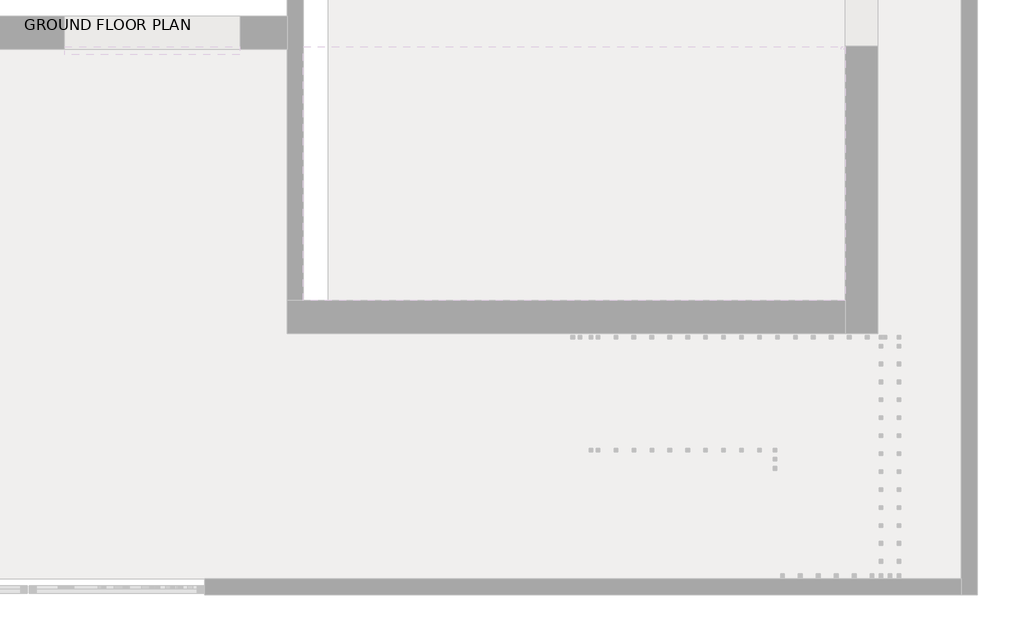
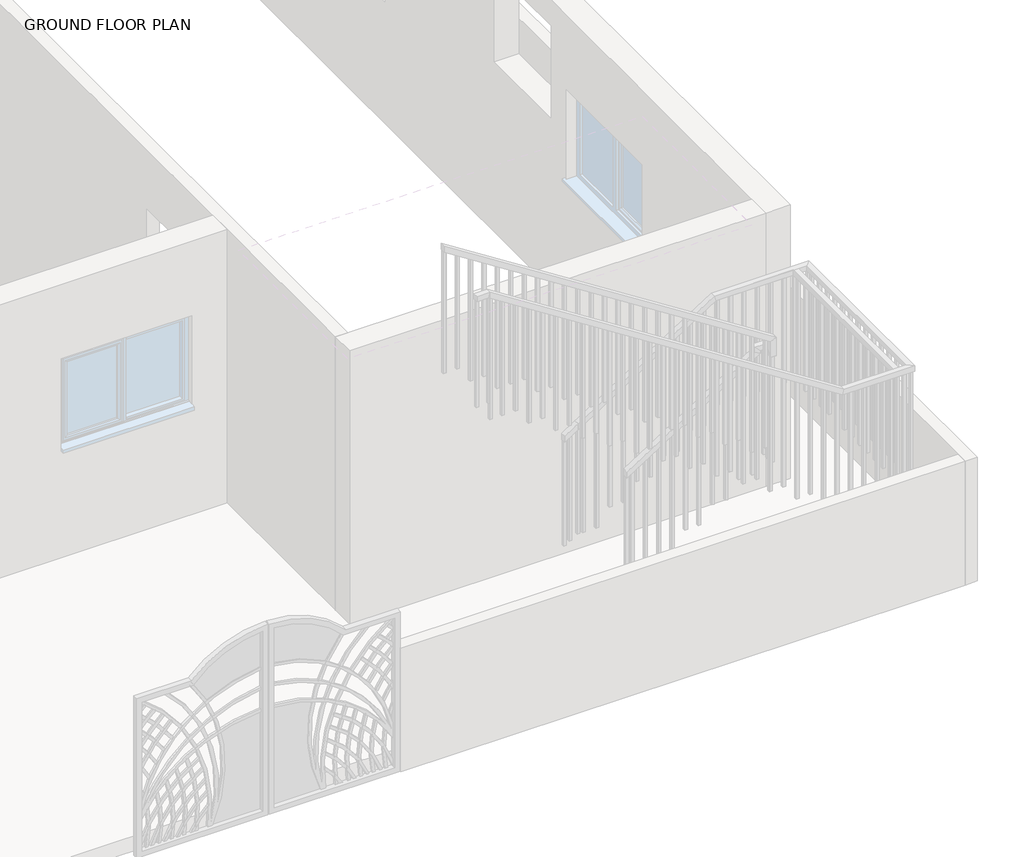
# One storey, part 21 of 23: 2 railings.
"""IFC4 building model written with IfcOpenShell, lengths in millimetres."""

from ifc_helpers import new_model, si_unit, frame, origin, place, context, project, spatial, polyline, outline, extrude, faceted_brep, element, save

model = new_model("IFC4")

# Units and contexts
model_context = context("Model", 3, world=origin())
ifc_project = project(units=[si_unit("LENGTHUNIT", "METRE", prefix="MILLI")], contexts=[model_context])

# Site, building, storey
site = spatial("IfcSite", under=ifc_project)
building = spatial("IfcBuilding", under=site)
storey = spatial("IfcBuildingStorey", under=building, Name="GROUND FLOOR PLAN", Elevation=487.68)

# Railings
placement = place(None, origin())
element("IfcRailing", 1, ObjectType="1100mm", at=placement, inside=storey, context=model_context, shape_type="SolidModel", body=[
    faceted_brep([(-8680.149573, -10220.0521308, 1912.8), (-8680.149573, -10220.0521308, 1853.4423995), (-8680.149573, -10270.0521308, 1853.4423995), (-8680.149573, -10270.0521308, 1912.8), (-7409.7306254, -10220.0521308, 2725.6), (-7395.1045513, -10220.0521308, 2675.6), (-7395.1045513, -10270.0521308, 2675.6), (-7409.7306254, -10270.0521308, 2725.6), (-6495.8132565, -10220.0521308, 2725.6), (-6495.8132565, -10220.0521308, 2675.6), (-6545.8132565, -10270.0521308, 2675.6), (-6545.8132565, -10270.0521308, 2725.6), (-6495.8132565, -11933.6860066, 2725.6), (-6495.8132565, -11933.6860066, 2675.6), (-6545.8132565, -11883.6860066, 2675.6), (-6545.8132565, -11883.6860066, 2725.6), (-7155.718398, -11933.6860066, 2725.6), (-7170.3479429, -11933.6860066, 2675.6), (-7170.3479429, -11883.6860066, 2675.6), (-7155.718398, -11883.6860066, 2725.6), (-10457.8773536, -11933.6860066, 4838.88), (-10457.8773536, -11883.6860066, 4838.88), (-10457.8773536, -11883.6860066, 4779.517542), (-10457.8773536, -11933.6860066, 4779.517542)], [[[0, 1, 2, 3]], [[1, 0, 4, 5]], [[2, 1, 5, 6]], [[3, 2, 6, 7]], [[0, 3, 7, 4]], [[5, 4, 8, 9]], [[6, 5, 9, 10]], [[7, 6, 10, 11]], [[4, 7, 11, 8]], [[9, 8, 12, 13]], [[10, 9, 13, 14]], [[11, 10, 14, 15]], [[8, 11, 15, 12]], [[13, 12, 16, 17]], [[14, 13, 17, 18]], [[15, 14, 18, 19]], [[12, 15, 19, 16]], [[20, 21, 22, 23]], [[17, 16, 20, 23]], [[18, 17, 23, 22]], [[19, 18, 22, 21]], [[16, 19, 21, 20]]]),
    extrude(outline(polyline([(4691.8007425, -10320.8132565), (4707.7999723, -10345.8132565), (3576.32, -10345.8132565), (3576.32, -10320.8132565), (4691.8007425, -10320.8132565)])), frame((0.0, -11921.1860066, 0.0), z_axis=(0.0, 1.0, 0.0), x_axis=(0.0, 0.0, 1.0)), (0.0, 0.0, 1.0), 25.0),
    extrude(outline(polyline([(4611.8045935, -10195.8132565), (4627.8038233, -10220.8132565), (3576.32, -10220.8132565), (3576.32, -10195.8132565), (4611.8045935, -10195.8132565)])), frame((0.0, -11921.1860066, 0.0), z_axis=(0.0, 1.0, 0.0), x_axis=(0.0, 0.0, 1.0)), (0.0, 0.0, 1.0), 25.0),
    extrude(outline(polyline([(4531.8084444, -10070.8132565), (4547.8076742, -10095.8132565), (3413.76, -10095.8132565), (3413.76, -10070.8132565), (4531.8084444, -10070.8132565)])), frame((0.0, -11921.1860066, 0.0), z_axis=(0.0, 1.0, 0.0), x_axis=(0.0, 0.0, 1.0)), (0.0, 0.0, 1.0), 25.0),
    extrude(outline(polyline([(4451.8122954, -9945.8132565), (4467.8115252, -9970.8132565), (3413.76, -9970.8132565), (3413.76, -9945.8132565), (4451.8122954, -9945.8132565)])), frame((0.0, -11921.1860066, 0.0), z_axis=(0.0, 1.0, 0.0), x_axis=(0.0, 0.0, 1.0)), (0.0, 0.0, 1.0), 25.0),
    extrude(outline(polyline([(4371.8161463, -9820.8132565), (4387.8153761, -9845.8132565), (3251.2, -9845.8132565), (3251.2, -9820.8132565), (4371.8161463, -9820.8132565)])), frame((0.0, -11921.1860066, 0.0), z_axis=(0.0, 1.0, 0.0), x_axis=(0.0, 0.0, 1.0)), (0.0, 0.0, 1.0), 25.0),
    extrude(outline(polyline([(4291.8423995, -9695.8132565), (4307.8371231, -9720.8132565), (3251.2, -9720.8132565), (3251.2, -9695.8132565), (4291.8423995, -9695.8132565)])), frame((0.0, -11921.1860066, 0.0), z_axis=(0.0, 1.0, 0.0), x_axis=(0.0, 0.0, 1.0)), (0.0, 0.0, 1.0), 25.0),
    extrude(outline(polyline([(4211.8238482, -9570.8132565), (4227.823078, -9595.8132565), (3088.64, -9595.8132565), (3088.64, -9570.8132565), (4211.8238482, -9570.8132565)])), frame((0.0, -11921.1860066, 0.0), z_axis=(0.0, 1.0, 0.0), x_axis=(0.0, 0.0, 1.0)), (0.0, 0.0, 1.0), 25.0),
    extrude(outline(polyline([(4131.8276992, -9445.8132565), (4147.826929, -9470.8132565), (3088.64, -9470.8132565), (3088.64, -9445.8132565), (4131.8276992, -9445.8132565)])), frame((0.0, -11921.1860066, 0.0), z_axis=(0.0, 1.0, 0.0), x_axis=(0.0, 0.0, 1.0)), (0.0, 0.0, 1.0), 25.0),
    extrude(outline(polyline([(4051.8315501, -9320.8132565), (4067.8307799, -9345.8132565), (2926.08, -9345.8132565), (2926.08, -9320.8132565), (4051.8315501, -9320.8132565)])), frame((0.0, -11921.1860066, 0.0), z_axis=(0.0, 1.0, 0.0), x_axis=(0.0, 0.0, 1.0)), (0.0, 0.0, 1.0), 25.0),
    extrude(outline(polyline([(3971.835401, -9195.8132565), (3987.8346309, -9220.8132565), (2926.08, -9220.8132565), (2926.08, -9195.8132565), (3971.835401, -9195.8132565)])), frame((0.0, -11921.1860066, 0.0), z_axis=(0.0, 1.0, 0.0), x_axis=(0.0, 0.0, 1.0)), (0.0, 0.0, 1.0), 25.0),
    extrude(outline(polyline([(3891.839252, -9070.8132565), (3907.8384818, -9095.8132565), (2763.52, -9095.8132565), (2763.52, -9070.8132565), (3891.839252, -9070.8132565)])), frame((0.0, -11921.1860066, 0.0), z_axis=(0.0, 1.0, 0.0), x_axis=(0.0, 0.0, 1.0)), (0.0, 0.0, 1.0), 25.0),
    extrude(outline(polyline([(3811.8431029, -8945.8132565), (3827.8423328, -8970.8132565), (2763.52, -8970.8132565), (2763.52, -8945.8132565), (3811.8431029, -8945.8132565)])), frame((0.0, -11921.1860066, 0.0), z_axis=(0.0, 1.0, 0.0), x_axis=(0.0, 0.0, 1.0)), (0.0, 0.0, 1.0), 25.0),
    extrude(outline(polyline([(3731.8469539, -8820.8132565), (3747.8461837, -8845.8132565), (2600.96, -8845.8132565), (2600.96, -8820.8132565), (3731.8469539, -8820.8132565)])), frame((0.0, -11921.1860066, 0.0), z_axis=(0.0, 1.0, 0.0), x_axis=(0.0, 0.0, 1.0)), (0.0, 0.0, 1.0), 25.0),
    extrude(outline(polyline([(3651.8508048, -8695.8132565), (3667.8500347, -8720.8132565), (2600.96, -8720.8132565), (2600.96, -8695.8132565), (3651.8508048, -8695.8132565)])), frame((0.0, -11921.1860066, 0.0), z_axis=(0.0, 1.0, 0.0), x_axis=(0.0, 0.0, 1.0)), (0.0, 0.0, 1.0), 25.0),
    extrude(outline(polyline([(3571.8546558, -8570.8132565), (3587.8538856, -8595.8132565), (2438.4, -8595.8132565), (2438.4, -8570.8132565), (3571.8546558, -8570.8132565)])), frame((0.0, -11921.1860066, 0.0), z_axis=(0.0, 1.0, 0.0), x_axis=(0.0, 0.0, 1.0)), (0.0, 0.0, 1.0), 25.0),
    extrude(outline(polyline([(3491.8585067, -8445.8132565), (3507.8577365, -8470.8132565), (2438.4, -8470.8132565), (2438.4, -8445.8132565), (3491.8585067, -8445.8132565)])), frame((0.0, -11921.1860066, 0.0), z_axis=(0.0, 1.0, 0.0), x_axis=(0.0, 0.0, 1.0)), (0.0, 0.0, 1.0), 25.0),
    extrude(outline(polyline([(3411.8623577, -8320.8132565), (3427.8615875, -8345.8132565), (2275.84, -8345.8132565), (2275.84, -8320.8132565), (3411.8623577, -8320.8132565)])), frame((0.0, -11921.1860066, 0.0), z_axis=(0.0, 1.0, 0.0), x_axis=(0.0, 0.0, 1.0)), (0.0, 0.0, 1.0), 25.0),
    extrude(outline(polyline([(3331.8662086, -8195.8132565), (3347.8654384, -8220.8132565), (2275.84, -8220.8132565), (2275.84, -8195.8132565), (3331.8662086, -8195.8132565)])), frame((0.0, -11921.1860066, 0.0), z_axis=(0.0, 1.0, 0.0), x_axis=(0.0, 0.0, 1.0)), (0.0, 0.0, 1.0), 25.0),
    extrude(outline(polyline([(3251.8700596, -8070.8132565), (3267.8692894, -8095.8132565), (2113.28, -8095.8132565), (2113.28, -8070.8132565), (3251.8700596, -8070.8132565)])), frame((0.0, -11921.1860066, 0.0), z_axis=(0.0, 1.0, 0.0), x_axis=(0.0, 0.0, 1.0)), (0.0, 0.0, 1.0), 25.0),
    extrude(outline(polyline([(3171.8739105, -7945.8132565), (3187.8731403, -7970.8132565), (2113.28, -7970.8132565), (2113.28, -7945.8132565), (3171.8739105, -7945.8132565)])), frame((0.0, -11921.1860066, 0.0), z_axis=(0.0, 1.0, 0.0), x_axis=(0.0, 0.0, 1.0)), (0.0, 0.0, 1.0), 25.0),
    extrude(outline(polyline([(3091.8777615, -7820.8132565), (3107.8769913, -7845.8132565), (1950.72, -7845.8132565), (1950.72, -7820.8132565), (3091.8777615, -7820.8132565)])), frame((0.0, -11921.1860066, 0.0), z_axis=(0.0, 1.0, 0.0), x_axis=(0.0, 0.0, 1.0)), (0.0, 0.0, 1.0), 25.0),
    extrude(outline(polyline([(3011.8816124, -7695.8132565), (3027.8808422, -7720.8132565), (1950.72, -7720.8132565), (1950.72, -7695.8132565), (3011.8816124, -7695.8132565)])), frame((0.0, -11921.1860066, 0.0), z_axis=(0.0, 1.0, 0.0), x_axis=(0.0, 0.0, 1.0)), (0.0, 0.0, 1.0), 25.0),
    extrude(outline(polyline([(2931.8854634, -7570.8132565), (2947.8846932, -7595.8132565), (1788.16, -7595.8132565), (1788.16, -7570.8132565), (2931.8854634, -7570.8132565)])), frame((0.0, -11921.1860066, 0.0), z_axis=(0.0, 1.0, 0.0), x_axis=(0.0, 0.0, 1.0)), (0.0, 0.0, 1.0), 25.0),
    extrude(outline(polyline([(2851.8893143, -7445.8132565), (2867.8885441, -7470.8132565), (1788.16, -7470.8132565), (1788.16, -7445.8132565), (2851.8893143, -7445.8132565)])), frame((0.0, -11921.1860066, 0.0), z_axis=(0.0, 1.0, 0.0), x_axis=(0.0, 0.0, 1.0)), (0.0, 0.0, 1.0), 25.0),
    extrude(outline(polyline([(2771.8931653, -7320.8132565), (2787.8923951, -7345.8132565), (1625.6, -7345.8132565), (1625.6, -7320.8132565), (2771.8931653, -7320.8132565)])), frame((0.0, -11921.1860066, 0.0), z_axis=(0.0, 1.0, 0.0), x_axis=(0.0, 0.0, 1.0)), (0.0, 0.0, 1.0), 25.0),
    extrude(outline(polyline([(2691.8970162, -7195.8132565), (2707.896246, -7220.8132565), (1625.6, -7220.8132565), (1625.6, -7195.8132565), (2691.8970162, -7195.8132565)])), frame((0.0, -11921.1860066, 0.0), z_axis=(0.0, 1.0, 0.0), x_axis=(0.0, 0.0, 1.0)), (0.0, 0.0, 1.0), 25.0),
    extrude(outline(polyline([(-7070.8132565, -11921.1860066), (-7095.8132565, -11921.1860066), (-7095.8132565, -11896.1860066), (-7070.8132565, -11896.1860066), (-7070.8132565, -11921.1860066)])), frame((0.0, 0.0, 1625.6), z_axis=(0.0, 0.0, 1.0), x_axis=(1.0, 0.0, 0.0)), (0.0, 0.0, 1.0), 1050.0),
    extrude(outline(polyline([(-6945.8132565, -11921.1860066), (-6970.8132565, -11921.1860066), (-6970.8132565, -11896.1860066), (-6945.8132565, -11896.1860066), (-6945.8132565, -11921.1860066)])), frame((0.0, 0.0, 1625.6), z_axis=(0.0, 0.0, 1.0), x_axis=(1.0, 0.0, 0.0)), (0.0, 0.0, 1.0), 1050.0),
    extrude(outline(polyline([(-6820.8132565, -11921.1860066), (-6845.8132565, -11921.1860066), (-6845.8132565, -11896.1860066), (-6820.8132565, -11896.1860066), (-6820.8132565, -11921.1860066)])), frame((0.0, 0.0, 1625.6), z_axis=(0.0, 0.0, 1.0), x_axis=(1.0, 0.0, 0.0)), (0.0, 0.0, 1.0), 1050.0),
    extrude(outline(polyline([(-6695.8132565, -11921.1860066), (-6720.8132565, -11921.1860066), (-6720.8132565, -11896.1860066), (-6695.8132565, -11896.1860066), (-6695.8132565, -11921.1860066)])), frame((0.0, 0.0, 1625.6), z_axis=(0.0, 0.0, 1.0), x_axis=(1.0, 0.0, 0.0)), (0.0, 0.0, 1.0), 1050.0),
    extrude(outline(polyline([(-6570.8132565, -11921.1860066), (-6595.8132565, -11921.1860066), (-6595.8132565, -11896.1860066), (-6570.8132565, -11896.1860066), (-6570.8132565, -11921.1860066)])), frame((0.0, 0.0, 1625.6), z_axis=(0.0, 0.0, 1.0), x_axis=(1.0, 0.0, 0.0)), (0.0, 0.0, 1.0), 1050.0),
    extrude(outline(polyline([(-6508.3132565, -11795.0521308), (-6508.3132565, -11820.0521308), (-6533.3132565, -11820.0521308), (-6533.3132565, -11795.0521308), (-6508.3132565, -11795.0521308)])), frame((0.0, 0.0, 1625.6), z_axis=(0.0, 0.0, 1.0), x_axis=(1.0, 0.0, 0.0)), (0.0, 0.0, 1.0), 1050.0),
    extrude(outline(polyline([(-6508.3132565, -11670.0521308), (-6508.3132565, -11695.0521308), (-6533.3132565, -11695.0521308), (-6533.3132565, -11670.0521308), (-6508.3132565, -11670.0521308)])), frame((0.0, 0.0, 1625.6), z_axis=(0.0, 0.0, 1.0), x_axis=(1.0, 0.0, 0.0)), (0.0, 0.0, 1.0), 1050.0),
    extrude(outline(polyline([(-6508.3132565, -11545.0521308), (-6508.3132565, -11570.0521308), (-6533.3132565, -11570.0521308), (-6533.3132565, -11545.0521308), (-6508.3132565, -11545.0521308)])), frame((0.0, 0.0, 1625.6), z_axis=(0.0, 0.0, 1.0), x_axis=(1.0, 0.0, 0.0)), (0.0, 0.0, 1.0), 1050.0),
    extrude(outline(polyline([(-6508.3132565, -11420.0521308), (-6508.3132565, -11445.0521308), (-6533.3132565, -11445.0521308), (-6533.3132565, -11420.0521308), (-6508.3132565, -11420.0521308)])), frame((0.0, 0.0, 1625.6), z_axis=(0.0, 0.0, 1.0), x_axis=(1.0, 0.0, 0.0)), (0.0, 0.0, 1.0), 1050.0),
    extrude(outline(polyline([(-6508.3132565, -11295.0521308), (-6508.3132565, -11320.0521308), (-6533.3132565, -11320.0521308), (-6533.3132565, -11295.0521308), (-6508.3132565, -11295.0521308)])), frame((0.0, 0.0, 1625.6), z_axis=(0.0, 0.0, 1.0), x_axis=(1.0, 0.0, 0.0)), (0.0, 0.0, 1.0), 1050.0),
    extrude(outline(polyline([(-6508.3132565, -11170.0521308), (-6508.3132565, -11195.0521308), (-6533.3132565, -11195.0521308), (-6533.3132565, -11170.0521308), (-6508.3132565, -11170.0521308)])), frame((0.0, 0.0, 1625.6), z_axis=(0.0, 0.0, 1.0), x_axis=(1.0, 0.0, 0.0)), (0.0, 0.0, 1.0), 1050.0),
    extrude(outline(polyline([(-6508.3132565, -11045.0521308), (-6508.3132565, -11070.0521308), (-6533.3132565, -11070.0521308), (-6533.3132565, -11045.0521308), (-6508.3132565, -11045.0521308)])), frame((0.0, 0.0, 1625.6), z_axis=(0.0, 0.0, 1.0), x_axis=(1.0, 0.0, 0.0)), (0.0, 0.0, 1.0), 1050.0),
    extrude(outline(polyline([(-6508.3132565, -10920.0521308), (-6508.3132565, -10945.0521308), (-6533.3132565, -10945.0521308), (-6533.3132565, -10920.0521308), (-6508.3132565, -10920.0521308)])), frame((0.0, 0.0, 1625.6), z_axis=(0.0, 0.0, 1.0), x_axis=(1.0, 0.0, 0.0)), (0.0, 0.0, 1.0), 1050.0),
    extrude(outline(polyline([(-6508.3132565, -10795.0521308), (-6508.3132565, -10820.0521308), (-6533.3132565, -10820.0521308), (-6533.3132565, -10795.0521308), (-6508.3132565, -10795.0521308)])), frame((0.0, 0.0, 1625.6), z_axis=(0.0, 0.0, 1.0), x_axis=(1.0, 0.0, 0.0)), (0.0, 0.0, 1.0), 1050.0),
    extrude(outline(polyline([(-6508.3132565, -10670.0521308), (-6508.3132565, -10695.0521308), (-6533.3132565, -10695.0521308), (-6533.3132565, -10670.0521308), (-6508.3132565, -10670.0521308)])), frame((0.0, 0.0, 1625.6), z_axis=(0.0, 0.0, 1.0), x_axis=(1.0, 0.0, 0.0)), (0.0, 0.0, 1.0), 1050.0),
    extrude(outline(polyline([(-6508.3132565, -10545.0521308), (-6508.3132565, -10570.0521308), (-6533.3132565, -10570.0521308), (-6533.3132565, -10545.0521308), (-6508.3132565, -10545.0521308)])), frame((0.0, 0.0, 1625.6), z_axis=(0.0, 0.0, 1.0), x_axis=(1.0, 0.0, 0.0)), (0.0, 0.0, 1.0), 1050.0),
    extrude(outline(polyline([(-6508.3132565, -10420.0521308), (-6508.3132565, -10445.0521308), (-6533.3132565, -10445.0521308), (-6533.3132565, -10420.0521308), (-6508.3132565, -10420.0521308)])), frame((0.0, 0.0, 1625.6), z_axis=(0.0, 0.0, 1.0), x_axis=(1.0, 0.0, 0.0)), (0.0, 0.0, 1.0), 1050.0),
    extrude(outline(polyline([(-6508.3132565, -10295.0521308), (-6508.3132565, -10320.0521308), (-6533.3132565, -10320.0521308), (-6533.3132565, -10295.0521308), (-6508.3132565, -10295.0521308)])), frame((0.0, 0.0, 1625.6), z_axis=(0.0, 0.0, 1.0), x_axis=(1.0, 0.0, 0.0)), (0.0, 0.0, 1.0), 1050.0),
    extrude(outline(polyline([(-6630.149573, -10232.5521308), (-6605.149573, -10232.5521308), (-6605.149573, -10257.5521308), (-6630.149573, -10257.5521308), (-6630.149573, -10232.5521308)])), frame((0.0, 0.0, 1625.6), z_axis=(0.0, 0.0, 1.0), x_axis=(1.0, 0.0, 0.0)), (0.0, 0.0, 1.0), 1050.0),
    extrude(outline(polyline([(-6755.149573, -10232.5521308), (-6730.149573, -10232.5521308), (-6730.149573, -10257.5521308), (-6755.149573, -10257.5521308), (-6755.149573, -10232.5521308)])), frame((0.0, 0.0, 1625.6), z_axis=(0.0, 0.0, 1.0), x_axis=(1.0, 0.0, 0.0)), (0.0, 0.0, 1.0), 1050.0),
    extrude(outline(polyline([(-6880.149573, -10232.5521308), (-6855.149573, -10232.5521308), (-6855.149573, -10257.5521308), (-6880.149573, -10257.5521308), (-6880.149573, -10232.5521308)])), frame((0.0, 0.0, 1625.6), z_axis=(0.0, 0.0, 1.0), x_axis=(1.0, 0.0, 0.0)), (0.0, 0.0, 1.0), 1050.0),
    extrude(outline(polyline([(-7005.149573, -10232.5521308), (-6980.149573, -10232.5521308), (-6980.149573, -10257.5521308), (-7005.149573, -10257.5521308), (-7005.149573, -10232.5521308)])), frame((0.0, 0.0, 1625.6), z_axis=(0.0, 0.0, 1.0), x_axis=(1.0, 0.0, 0.0)), (0.0, 0.0, 1.0), 1050.0),
    extrude(outline(polyline([(-7130.149573, -10232.5521308), (-7105.149573, -10232.5521308), (-7105.149573, -10257.5521308), (-7130.149573, -10257.5521308), (-7130.149573, -10232.5521308)])), frame((0.0, 0.0, 1625.6), z_axis=(0.0, 0.0, 1.0), x_axis=(1.0, 0.0, 0.0)), (0.0, 0.0, 1.0), 1050.0),
    extrude(outline(polyline([(-7255.149573, -10232.5521308), (-7230.149573, -10232.5521308), (-7230.149573, -10257.5521308), (-7255.149573, -10257.5521308), (-7255.149573, -10232.5521308)])), frame((0.0, 0.0, 1625.6), z_axis=(0.0, 0.0, 1.0), x_axis=(1.0, 0.0, 0.0)), (0.0, 0.0, 1.0), 1050.0),
    extrude(outline(polyline([(-7380.149573, -10232.5521308), (-7355.149573, -10232.5521308), (-7355.149573, -10257.5521308), (-7380.149573, -10257.5521308), (-7380.149573, -10232.5521308)])), frame((0.0, 0.0, 1625.6), z_axis=(0.0, 0.0, 1.0), x_axis=(1.0, 0.0, 0.0)), (0.0, 0.0, 1.0), 1050.0),
    extrude(outline(polyline([(1463.04, -7505.149573), (1463.04, -7480.149573), (2621.1891352, -7480.149573), (2605.1944115, -7505.149573), (1463.04, -7505.149573)])), frame((0.0, -10257.5521308, 0.0), z_axis=(0.0, 1.0, 0.0), x_axis=(0.0, 0.0, 1.0)), (0.0, 0.0, 1.0), 25.0),
    extrude(outline(polyline([(1463.04, -7630.149573), (1463.04, -7605.149573), (2541.2155169, -7605.149573), (2525.2207932, -7630.149573), (1463.04, -7630.149573)])), frame((0.0, -10257.5521308, 0.0), z_axis=(0.0, 1.0, 0.0), x_axis=(0.0, 0.0, 1.0)), (0.0, 0.0, 1.0), 25.0),
    extrude(outline(polyline([(1300.48, -7755.149573), (1300.48, -7730.149573), (2461.2418986, -7730.149573), (2445.2471749, -7755.149573), (1300.48, -7755.149573)])), frame((0.0, -10257.5521308, 0.0), z_axis=(0.0, 1.0, 0.0), x_axis=(0.0, 0.0, 1.0)), (0.0, 0.0, 1.0), 25.0),
    extrude(outline(polyline([(1300.48, -7880.149573), (1300.48, -7855.149573), (2381.2682803, -7855.149573), (2365.2735566, -7880.149573), (1300.48, -7880.149573)])), frame((0.0, -10257.5521308, 0.0), z_axis=(0.0, 1.0, 0.0), x_axis=(0.0, 0.0, 1.0)), (0.0, 0.0, 1.0), 25.0),
    extrude(outline(polyline([(1137.92, -8005.149573), (1137.92, -7980.149573), (2301.294662, -7980.149573), (2285.2999383, -8005.149573), (1137.92, -8005.149573)])), frame((0.0, -10257.5521308, 0.0), z_axis=(0.0, 1.0, 0.0), x_axis=(0.0, 0.0, 1.0)), (0.0, 0.0, 1.0), 25.0),
    extrude(outline(polyline([(1137.92, -8130.149573), (1137.92, -8105.149573), (2221.3210437, -8105.149573), (2205.32632, -8130.149573), (1137.92, -8130.149573)])), frame((0.0, -10257.5521308, 0.0), z_axis=(0.0, 1.0, 0.0), x_axis=(0.0, 0.0, 1.0)), (0.0, 0.0, 1.0), 25.0),
    extrude(outline(polyline([(975.36, -8255.149573), (975.36, -8230.149573), (2141.3474254, -8230.149573), (2125.3527017, -8255.149573), (975.36, -8255.149573)])), frame((0.0, -10257.5521308, 0.0), z_axis=(0.0, 1.0, 0.0), x_axis=(0.0, 0.0, 1.0)), (0.0, 0.0, 1.0), 25.0),
    extrude(outline(polyline([(975.36, -8380.149573), (975.36, -8355.149573), (2061.3738071, -8355.149573), (2045.3790834, -8380.149573), (975.36, -8380.149573)])), frame((0.0, -10257.5521308, 0.0), z_axis=(0.0, 1.0, 0.0), x_axis=(0.0, 0.0, 1.0)), (0.0, 0.0, 1.0), 25.0),
    extrude(outline(polyline([(812.8, -8505.149573), (812.8, -8480.149573), (1981.4001888, -8480.149573), (1965.4054651, -8505.149573), (812.8, -8505.149573)])), frame((0.0, -10257.5521308, 0.0), z_axis=(0.0, 1.0, 0.0), x_axis=(0.0, 0.0, 1.0)), (0.0, 0.0, 1.0), 25.0),
    extrude(outline(polyline([(812.8, -8630.149573), (812.8, -8605.149573), (1901.4265705, -8605.149573), (1885.4318468, -8630.149573), (812.8, -8630.149573)])), frame((0.0, -10257.5521308, 0.0), z_axis=(0.0, 1.0, 0.0), x_axis=(0.0, 0.0, 1.0)), (0.0, 0.0, 1.0), 25.0),
    extrude(outline(polyline([(-6508.3132565, -11896.1860066), (-6508.3132565, -11921.1860066), (-6533.3132565, -11921.1860066), (-6533.3132565, -11896.1860066), (-6508.3132565, -11896.1860066)])), frame((0.0, 0.0, 1625.6), z_axis=(0.0, 0.0, 1.0), x_axis=(1.0, 0.0, 0.0)), (0.0, 0.0, 1.0), 1050.0),
    extrude(outline(polyline([(-6533.3132565, -10232.5521308), (-6508.3132565, -10232.5521308), (-6508.3132565, -10257.5521308), (-6533.3132565, -10257.5521308), (-6533.3132565, -10232.5521308)])), frame((0.0, 0.0, 1625.6), z_axis=(0.0, 0.0, 1.0), x_axis=(1.0, 0.0, 0.0)), (0.0, 0.0, 1.0), 1050.0),
    extrude(outline(polyline([(4763.5183122, -10432.8773536), (4779.517542, -10457.8773536), (3576.32, -10457.8773536), (3576.32, -10432.8773536), (4763.5183122, -10432.8773536)])), frame((0.0, -11921.1860066, 0.0), z_axis=(0.0, 1.0, 0.0), x_axis=(0.0, 0.0, 1.0)), (0.0, 0.0, 1.0), 25.0),
    extrude(outline(polyline([(812.8, -8680.149573), (812.8, -8655.149573), (1869.4371231, -8655.149573), (1853.4423995, -8680.149573), (812.8, -8680.149573)])), frame((0.0, -10257.5521308, 0.0), z_axis=(0.0, 1.0, 0.0), x_axis=(0.0, 0.0, 1.0)), (0.0, 0.0, 1.0), 25.0),
])
element("IfcRailing", 2, ObjectType="1100mm", at=placement, inside=storey, context=model_context, shape_type="SolidModel", body=[
    faceted_brep([(-8680.149573, -10220.0521308, 1912.8), (-8680.149573, -10220.0521308, 1853.4423995), (-8680.149573, -10270.0521308, 1853.4423995), (-8680.149573, -10270.0521308, 1912.8), (-7409.7306254, -10220.0521308, 2725.6), (-7395.1045513, -10220.0521308, 2675.6), (-7395.1045513, -10270.0521308, 2675.6), (-7409.7306254, -10270.0521308, 2725.6), (-6495.8132565, -10220.0521308, 2725.6), (-6495.8132565, -10220.0521308, 2675.6), (-6545.8132565, -10270.0521308, 2675.6), (-6545.8132565, -10270.0521308, 2725.6), (-6495.8132565, -11933.6860066, 2725.6), (-6495.8132565, -11933.6860066, 2675.6), (-6545.8132565, -11883.6860066, 2675.6), (-6545.8132565, -11883.6860066, 2725.6), (-7155.718398, -11933.6860066, 2725.6), (-7170.3479429, -11933.6860066, 2675.6), (-7170.3479429, -11883.6860066, 2675.6), (-7155.718398, -11883.6860066, 2725.6), (-10457.8773536, -11933.6860066, 4838.88), (-10457.8773536, -11883.6860066, 4838.88), (-10457.8773536, -11883.6860066, 4779.517542), (-10457.8773536, -11933.6860066, 4779.517542)], [[[0, 1, 2, 3]], [[1, 0, 4, 5]], [[2, 1, 5, 6]], [[3, 2, 6, 7]], [[0, 3, 7, 4]], [[5, 4, 8, 9]], [[6, 5, 9, 10]], [[7, 6, 10, 11]], [[4, 7, 11, 8]], [[9, 8, 12, 13]], [[10, 9, 13, 14]], [[11, 10, 14, 15]], [[8, 11, 15, 12]], [[13, 12, 16, 17]], [[14, 13, 17, 18]], [[15, 14, 18, 19]], [[12, 15, 19, 16]], [[20, 21, 22, 23]], [[17, 16, 20, 23]], [[18, 17, 23, 22]], [[19, 18, 22, 21]], [[16, 19, 21, 20]]]),
    extrude(outline(polyline([(4691.8007425, -10320.8132565), (4707.7999723, -10345.8132565), (3576.32, -10345.8132565), (3576.32, -10320.8132565), (4691.8007425, -10320.8132565)])), frame((0.0, -11921.1860066, 0.0), z_axis=(0.0, 1.0, 0.0), x_axis=(0.0, 0.0, 1.0)), (0.0, 0.0, 1.0), 25.0),
    extrude(outline(polyline([(4611.8045935, -10195.8132565), (4627.8038233, -10220.8132565), (3576.32, -10220.8132565), (3576.32, -10195.8132565), (4611.8045935, -10195.8132565)])), frame((0.0, -11921.1860066, 0.0), z_axis=(0.0, 1.0, 0.0), x_axis=(0.0, 0.0, 1.0)), (0.0, 0.0, 1.0), 25.0),
    extrude(outline(polyline([(4531.8084444, -10070.8132565), (4547.8076742, -10095.8132565), (3413.76, -10095.8132565), (3413.76, -10070.8132565), (4531.8084444, -10070.8132565)])), frame((0.0, -11921.1860066, 0.0), z_axis=(0.0, 1.0, 0.0), x_axis=(0.0, 0.0, 1.0)), (0.0, 0.0, 1.0), 25.0),
    extrude(outline(polyline([(4451.8122954, -9945.8132565), (4467.8115252, -9970.8132565), (3413.76, -9970.8132565), (3413.76, -9945.8132565), (4451.8122954, -9945.8132565)])), frame((0.0, -11921.1860066, 0.0), z_axis=(0.0, 1.0, 0.0), x_axis=(0.0, 0.0, 1.0)), (0.0, 0.0, 1.0), 25.0),
    extrude(outline(polyline([(4371.8161463, -9820.8132565), (4387.8153761, -9845.8132565), (3251.2, -9845.8132565), (3251.2, -9820.8132565), (4371.8161463, -9820.8132565)])), frame((0.0, -11921.1860066, 0.0), z_axis=(0.0, 1.0, 0.0), x_axis=(0.0, 0.0, 1.0)), (0.0, 0.0, 1.0), 25.0),
    extrude(outline(polyline([(4291.8423995, -9695.8132565), (4307.8371231, -9720.8132565), (3251.2, -9720.8132565), (3251.2, -9695.8132565), (4291.8423995, -9695.8132565)])), frame((0.0, -11921.1860066, 0.0), z_axis=(0.0, 1.0, 0.0), x_axis=(0.0, 0.0, 1.0)), (0.0, 0.0, 1.0), 25.0),
    extrude(outline(polyline([(4211.8238482, -9570.8132565), (4227.823078, -9595.8132565), (3088.64, -9595.8132565), (3088.64, -9570.8132565), (4211.8238482, -9570.8132565)])), frame((0.0, -11921.1860066, 0.0), z_axis=(0.0, 1.0, 0.0), x_axis=(0.0, 0.0, 1.0)), (0.0, 0.0, 1.0), 25.0),
    extrude(outline(polyline([(4131.8276992, -9445.8132565), (4147.826929, -9470.8132565), (3088.64, -9470.8132565), (3088.64, -9445.8132565), (4131.8276992, -9445.8132565)])), frame((0.0, -11921.1860066, 0.0), z_axis=(0.0, 1.0, 0.0), x_axis=(0.0, 0.0, 1.0)), (0.0, 0.0, 1.0), 25.0),
    extrude(outline(polyline([(4051.8315501, -9320.8132565), (4067.8307799, -9345.8132565), (2926.08, -9345.8132565), (2926.08, -9320.8132565), (4051.8315501, -9320.8132565)])), frame((0.0, -11921.1860066, 0.0), z_axis=(0.0, 1.0, 0.0), x_axis=(0.0, 0.0, 1.0)), (0.0, 0.0, 1.0), 25.0),
    extrude(outline(polyline([(3971.835401, -9195.8132565), (3987.8346309, -9220.8132565), (2926.08, -9220.8132565), (2926.08, -9195.8132565), (3971.835401, -9195.8132565)])), frame((0.0, -11921.1860066, 0.0), z_axis=(0.0, 1.0, 0.0), x_axis=(0.0, 0.0, 1.0)), (0.0, 0.0, 1.0), 25.0),
    extrude(outline(polyline([(3891.839252, -9070.8132565), (3907.8384818, -9095.8132565), (2763.52, -9095.8132565), (2763.52, -9070.8132565), (3891.839252, -9070.8132565)])), frame((0.0, -11921.1860066, 0.0), z_axis=(0.0, 1.0, 0.0), x_axis=(0.0, 0.0, 1.0)), (0.0, 0.0, 1.0), 25.0),
    extrude(outline(polyline([(3811.8431029, -8945.8132565), (3827.8423328, -8970.8132565), (2763.52, -8970.8132565), (2763.52, -8945.8132565), (3811.8431029, -8945.8132565)])), frame((0.0, -11921.1860066, 0.0), z_axis=(0.0, 1.0, 0.0), x_axis=(0.0, 0.0, 1.0)), (0.0, 0.0, 1.0), 25.0),
    extrude(outline(polyline([(3731.8469539, -8820.8132565), (3747.8461837, -8845.8132565), (2600.96, -8845.8132565), (2600.96, -8820.8132565), (3731.8469539, -8820.8132565)])), frame((0.0, -11921.1860066, 0.0), z_axis=(0.0, 1.0, 0.0), x_axis=(0.0, 0.0, 1.0)), (0.0, 0.0, 1.0), 25.0),
    extrude(outline(polyline([(3651.8508048, -8695.8132565), (3667.8500347, -8720.8132565), (2600.96, -8720.8132565), (2600.96, -8695.8132565), (3651.8508048, -8695.8132565)])), frame((0.0, -11921.1860066, 0.0), z_axis=(0.0, 1.0, 0.0), x_axis=(0.0, 0.0, 1.0)), (0.0, 0.0, 1.0), 25.0),
    extrude(outline(polyline([(3571.8546558, -8570.8132565), (3587.8538856, -8595.8132565), (2438.4, -8595.8132565), (2438.4, -8570.8132565), (3571.8546558, -8570.8132565)])), frame((0.0, -11921.1860066, 0.0), z_axis=(0.0, 1.0, 0.0), x_axis=(0.0, 0.0, 1.0)), (0.0, 0.0, 1.0), 25.0),
    extrude(outline(polyline([(3491.8585067, -8445.8132565), (3507.8577365, -8470.8132565), (2438.4, -8470.8132565), (2438.4, -8445.8132565), (3491.8585067, -8445.8132565)])), frame((0.0, -11921.1860066, 0.0), z_axis=(0.0, 1.0, 0.0), x_axis=(0.0, 0.0, 1.0)), (0.0, 0.0, 1.0), 25.0),
    extrude(outline(polyline([(3411.8623577, -8320.8132565), (3427.8615875, -8345.8132565), (2275.84, -8345.8132565), (2275.84, -8320.8132565), (3411.8623577, -8320.8132565)])), frame((0.0, -11921.1860066, 0.0), z_axis=(0.0, 1.0, 0.0), x_axis=(0.0, 0.0, 1.0)), (0.0, 0.0, 1.0), 25.0),
    extrude(outline(polyline([(3331.8662086, -8195.8132565), (3347.8654384, -8220.8132565), (2275.84, -8220.8132565), (2275.84, -8195.8132565), (3331.8662086, -8195.8132565)])), frame((0.0, -11921.1860066, 0.0), z_axis=(0.0, 1.0, 0.0), x_axis=(0.0, 0.0, 1.0)), (0.0, 0.0, 1.0), 25.0),
    extrude(outline(polyline([(3251.8700596, -8070.8132565), (3267.8692894, -8095.8132565), (2113.28, -8095.8132565), (2113.28, -8070.8132565), (3251.8700596, -8070.8132565)])), frame((0.0, -11921.1860066, 0.0), z_axis=(0.0, 1.0, 0.0), x_axis=(0.0, 0.0, 1.0)), (0.0, 0.0, 1.0), 25.0),
    extrude(outline(polyline([(3171.8739105, -7945.8132565), (3187.8731403, -7970.8132565), (2113.28, -7970.8132565), (2113.28, -7945.8132565), (3171.8739105, -7945.8132565)])), frame((0.0, -11921.1860066, 0.0), z_axis=(0.0, 1.0, 0.0), x_axis=(0.0, 0.0, 1.0)), (0.0, 0.0, 1.0), 25.0),
    extrude(outline(polyline([(3091.8777615, -7820.8132565), (3107.8769913, -7845.8132565), (1950.72, -7845.8132565), (1950.72, -7820.8132565), (3091.8777615, -7820.8132565)])), frame((0.0, -11921.1860066, 0.0), z_axis=(0.0, 1.0, 0.0), x_axis=(0.0, 0.0, 1.0)), (0.0, 0.0, 1.0), 25.0),
    extrude(outline(polyline([(3011.8816124, -7695.8132565), (3027.8808422, -7720.8132565), (1950.72, -7720.8132565), (1950.72, -7695.8132565), (3011.8816124, -7695.8132565)])), frame((0.0, -11921.1860066, 0.0), z_axis=(0.0, 1.0, 0.0), x_axis=(0.0, 0.0, 1.0)), (0.0, 0.0, 1.0), 25.0),
    extrude(outline(polyline([(2931.8854634, -7570.8132565), (2947.8846932, -7595.8132565), (1788.16, -7595.8132565), (1788.16, -7570.8132565), (2931.8854634, -7570.8132565)])), frame((0.0, -11921.1860066, 0.0), z_axis=(0.0, 1.0, 0.0), x_axis=(0.0, 0.0, 1.0)), (0.0, 0.0, 1.0), 25.0),
    extrude(outline(polyline([(2851.8893143, -7445.8132565), (2867.8885441, -7470.8132565), (1788.16, -7470.8132565), (1788.16, -7445.8132565), (2851.8893143, -7445.8132565)])), frame((0.0, -11921.1860066, 0.0), z_axis=(0.0, 1.0, 0.0), x_axis=(0.0, 0.0, 1.0)), (0.0, 0.0, 1.0), 25.0),
    extrude(outline(polyline([(2771.8931653, -7320.8132565), (2787.8923951, -7345.8132565), (1625.6, -7345.8132565), (1625.6, -7320.8132565), (2771.8931653, -7320.8132565)])), frame((0.0, -11921.1860066, 0.0), z_axis=(0.0, 1.0, 0.0), x_axis=(0.0, 0.0, 1.0)), (0.0, 0.0, 1.0), 25.0),
    extrude(outline(polyline([(2691.8970162, -7195.8132565), (2707.896246, -7220.8132565), (1625.6, -7220.8132565), (1625.6, -7195.8132565), (2691.8970162, -7195.8132565)])), frame((0.0, -11921.1860066, 0.0), z_axis=(0.0, 1.0, 0.0), x_axis=(0.0, 0.0, 1.0)), (0.0, 0.0, 1.0), 25.0),
    extrude(outline(polyline([(-7070.8132565, -11921.1860066), (-7095.8132565, -11921.1860066), (-7095.8132565, -11896.1860066), (-7070.8132565, -11896.1860066), (-7070.8132565, -11921.1860066)])), frame((0.0, 0.0, 1625.6), z_axis=(0.0, 0.0, 1.0), x_axis=(1.0, 0.0, 0.0)), (0.0, 0.0, 1.0), 1050.0),
    extrude(outline(polyline([(-6945.8132565, -11921.1860066), (-6970.8132565, -11921.1860066), (-6970.8132565, -11896.1860066), (-6945.8132565, -11896.1860066), (-6945.8132565, -11921.1860066)])), frame((0.0, 0.0, 1625.6), z_axis=(0.0, 0.0, 1.0), x_axis=(1.0, 0.0, 0.0)), (0.0, 0.0, 1.0), 1050.0),
    extrude(outline(polyline([(-6820.8132565, -11921.1860066), (-6845.8132565, -11921.1860066), (-6845.8132565, -11896.1860066), (-6820.8132565, -11896.1860066), (-6820.8132565, -11921.1860066)])), frame((0.0, 0.0, 1625.6), z_axis=(0.0, 0.0, 1.0), x_axis=(1.0, 0.0, 0.0)), (0.0, 0.0, 1.0), 1050.0),
    extrude(outline(polyline([(-6695.8132565, -11921.1860066), (-6720.8132565, -11921.1860066), (-6720.8132565, -11896.1860066), (-6695.8132565, -11896.1860066), (-6695.8132565, -11921.1860066)])), frame((0.0, 0.0, 1625.6), z_axis=(0.0, 0.0, 1.0), x_axis=(1.0, 0.0, 0.0)), (0.0, 0.0, 1.0), 1050.0),
    extrude(outline(polyline([(-6570.8132565, -11921.1860066), (-6595.8132565, -11921.1860066), (-6595.8132565, -11896.1860066), (-6570.8132565, -11896.1860066), (-6570.8132565, -11921.1860066)])), frame((0.0, 0.0, 1625.6), z_axis=(0.0, 0.0, 1.0), x_axis=(1.0, 0.0, 0.0)), (0.0, 0.0, 1.0), 1050.0),
    extrude(outline(polyline([(-6508.3132565, -11795.0521308), (-6508.3132565, -11820.0521308), (-6533.3132565, -11820.0521308), (-6533.3132565, -11795.0521308), (-6508.3132565, -11795.0521308)])), frame((0.0, 0.0, 1625.6), z_axis=(0.0, 0.0, 1.0), x_axis=(1.0, 0.0, 0.0)), (0.0, 0.0, 1.0), 1050.0),
    extrude(outline(polyline([(-6508.3132565, -11670.0521308), (-6508.3132565, -11695.0521308), (-6533.3132565, -11695.0521308), (-6533.3132565, -11670.0521308), (-6508.3132565, -11670.0521308)])), frame((0.0, 0.0, 1625.6), z_axis=(0.0, 0.0, 1.0), x_axis=(1.0, 0.0, 0.0)), (0.0, 0.0, 1.0), 1050.0),
    extrude(outline(polyline([(-6508.3132565, -11545.0521308), (-6508.3132565, -11570.0521308), (-6533.3132565, -11570.0521308), (-6533.3132565, -11545.0521308), (-6508.3132565, -11545.0521308)])), frame((0.0, 0.0, 1625.6), z_axis=(0.0, 0.0, 1.0), x_axis=(1.0, 0.0, 0.0)), (0.0, 0.0, 1.0), 1050.0),
    extrude(outline(polyline([(-6508.3132565, -11420.0521308), (-6508.3132565, -11445.0521308), (-6533.3132565, -11445.0521308), (-6533.3132565, -11420.0521308), (-6508.3132565, -11420.0521308)])), frame((0.0, 0.0, 1625.6), z_axis=(0.0, 0.0, 1.0), x_axis=(1.0, 0.0, 0.0)), (0.0, 0.0, 1.0), 1050.0),
    extrude(outline(polyline([(-6508.3132565, -11295.0521308), (-6508.3132565, -11320.0521308), (-6533.3132565, -11320.0521308), (-6533.3132565, -11295.0521308), (-6508.3132565, -11295.0521308)])), frame((0.0, 0.0, 1625.6), z_axis=(0.0, 0.0, 1.0), x_axis=(1.0, 0.0, 0.0)), (0.0, 0.0, 1.0), 1050.0),
    extrude(outline(polyline([(-6508.3132565, -11170.0521308), (-6508.3132565, -11195.0521308), (-6533.3132565, -11195.0521308), (-6533.3132565, -11170.0521308), (-6508.3132565, -11170.0521308)])), frame((0.0, 0.0, 1625.6), z_axis=(0.0, 0.0, 1.0), x_axis=(1.0, 0.0, 0.0)), (0.0, 0.0, 1.0), 1050.0),
    extrude(outline(polyline([(-6508.3132565, -11045.0521308), (-6508.3132565, -11070.0521308), (-6533.3132565, -11070.0521308), (-6533.3132565, -11045.0521308), (-6508.3132565, -11045.0521308)])), frame((0.0, 0.0, 1625.6), z_axis=(0.0, 0.0, 1.0), x_axis=(1.0, 0.0, 0.0)), (0.0, 0.0, 1.0), 1050.0),
    extrude(outline(polyline([(-6508.3132565, -10920.0521308), (-6508.3132565, -10945.0521308), (-6533.3132565, -10945.0521308), (-6533.3132565, -10920.0521308), (-6508.3132565, -10920.0521308)])), frame((0.0, 0.0, 1625.6), z_axis=(0.0, 0.0, 1.0), x_axis=(1.0, 0.0, 0.0)), (0.0, 0.0, 1.0), 1050.0),
    extrude(outline(polyline([(-6508.3132565, -10795.0521308), (-6508.3132565, -10820.0521308), (-6533.3132565, -10820.0521308), (-6533.3132565, -10795.0521308), (-6508.3132565, -10795.0521308)])), frame((0.0, 0.0, 1625.6), z_axis=(0.0, 0.0, 1.0), x_axis=(1.0, 0.0, 0.0)), (0.0, 0.0, 1.0), 1050.0),
    extrude(outline(polyline([(-6508.3132565, -10670.0521308), (-6508.3132565, -10695.0521308), (-6533.3132565, -10695.0521308), (-6533.3132565, -10670.0521308), (-6508.3132565, -10670.0521308)])), frame((0.0, 0.0, 1625.6), z_axis=(0.0, 0.0, 1.0), x_axis=(1.0, 0.0, 0.0)), (0.0, 0.0, 1.0), 1050.0),
    extrude(outline(polyline([(-6508.3132565, -10545.0521308), (-6508.3132565, -10570.0521308), (-6533.3132565, -10570.0521308), (-6533.3132565, -10545.0521308), (-6508.3132565, -10545.0521308)])), frame((0.0, 0.0, 1625.6), z_axis=(0.0, 0.0, 1.0), x_axis=(1.0, 0.0, 0.0)), (0.0, 0.0, 1.0), 1050.0),
    extrude(outline(polyline([(-6508.3132565, -10420.0521308), (-6508.3132565, -10445.0521308), (-6533.3132565, -10445.0521308), (-6533.3132565, -10420.0521308), (-6508.3132565, -10420.0521308)])), frame((0.0, 0.0, 1625.6), z_axis=(0.0, 0.0, 1.0), x_axis=(1.0, 0.0, 0.0)), (0.0, 0.0, 1.0), 1050.0),
    extrude(outline(polyline([(-6508.3132565, -10295.0521308), (-6508.3132565, -10320.0521308), (-6533.3132565, -10320.0521308), (-6533.3132565, -10295.0521308), (-6508.3132565, -10295.0521308)])), frame((0.0, 0.0, 1625.6), z_axis=(0.0, 0.0, 1.0), x_axis=(1.0, 0.0, 0.0)), (0.0, 0.0, 1.0), 1050.0),
    extrude(outline(polyline([(-6630.149573, -10232.5521308), (-6605.149573, -10232.5521308), (-6605.149573, -10257.5521308), (-6630.149573, -10257.5521308), (-6630.149573, -10232.5521308)])), frame((0.0, 0.0, 1625.6), z_axis=(0.0, 0.0, 1.0), x_axis=(1.0, 0.0, 0.0)), (0.0, 0.0, 1.0), 1050.0),
    extrude(outline(polyline([(-6755.149573, -10232.5521308), (-6730.149573, -10232.5521308), (-6730.149573, -10257.5521308), (-6755.149573, -10257.5521308), (-6755.149573, -10232.5521308)])), frame((0.0, 0.0, 1625.6), z_axis=(0.0, 0.0, 1.0), x_axis=(1.0, 0.0, 0.0)), (0.0, 0.0, 1.0), 1050.0),
    extrude(outline(polyline([(-6880.149573, -10232.5521308), (-6855.149573, -10232.5521308), (-6855.149573, -10257.5521308), (-6880.149573, -10257.5521308), (-6880.149573, -10232.5521308)])), frame((0.0, 0.0, 1625.6), z_axis=(0.0, 0.0, 1.0), x_axis=(1.0, 0.0, 0.0)), (0.0, 0.0, 1.0), 1050.0),
    extrude(outline(polyline([(-7005.149573, -10232.5521308), (-6980.149573, -10232.5521308), (-6980.149573, -10257.5521308), (-7005.149573, -10257.5521308), (-7005.149573, -10232.5521308)])), frame((0.0, 0.0, 1625.6), z_axis=(0.0, 0.0, 1.0), x_axis=(1.0, 0.0, 0.0)), (0.0, 0.0, 1.0), 1050.0),
    extrude(outline(polyline([(-7130.149573, -10232.5521308), (-7105.149573, -10232.5521308), (-7105.149573, -10257.5521308), (-7130.149573, -10257.5521308), (-7130.149573, -10232.5521308)])), frame((0.0, 0.0, 1625.6), z_axis=(0.0, 0.0, 1.0), x_axis=(1.0, 0.0, 0.0)), (0.0, 0.0, 1.0), 1050.0),
    extrude(outline(polyline([(-7255.149573, -10232.5521308), (-7230.149573, -10232.5521308), (-7230.149573, -10257.5521308), (-7255.149573, -10257.5521308), (-7255.149573, -10232.5521308)])), frame((0.0, 0.0, 1625.6), z_axis=(0.0, 0.0, 1.0), x_axis=(1.0, 0.0, 0.0)), (0.0, 0.0, 1.0), 1050.0),
    extrude(outline(polyline([(-7380.149573, -10232.5521308), (-7355.149573, -10232.5521308), (-7355.149573, -10257.5521308), (-7380.149573, -10257.5521308), (-7380.149573, -10232.5521308)])), frame((0.0, 0.0, 1625.6), z_axis=(0.0, 0.0, 1.0), x_axis=(1.0, 0.0, 0.0)), (0.0, 0.0, 1.0), 1050.0),
    extrude(outline(polyline([(1463.04, -7505.149573), (1463.04, -7480.149573), (2621.1891352, -7480.149573), (2605.1944115, -7505.149573), (1463.04, -7505.149573)])), frame((0.0, -10257.5521308, 0.0), z_axis=(0.0, 1.0, 0.0), x_axis=(0.0, 0.0, 1.0)), (0.0, 0.0, 1.0), 25.0),
    extrude(outline(polyline([(1463.04, -7630.149573), (1463.04, -7605.149573), (2541.2155169, -7605.149573), (2525.2207932, -7630.149573), (1463.04, -7630.149573)])), frame((0.0, -10257.5521308, 0.0), z_axis=(0.0, 1.0, 0.0), x_axis=(0.0, 0.0, 1.0)), (0.0, 0.0, 1.0), 25.0),
    extrude(outline(polyline([(1300.48, -7755.149573), (1300.48, -7730.149573), (2461.2418986, -7730.149573), (2445.2471749, -7755.149573), (1300.48, -7755.149573)])), frame((0.0, -10257.5521308, 0.0), z_axis=(0.0, 1.0, 0.0), x_axis=(0.0, 0.0, 1.0)), (0.0, 0.0, 1.0), 25.0),
    extrude(outline(polyline([(1300.48, -7880.149573), (1300.48, -7855.149573), (2381.2682803, -7855.149573), (2365.2735566, -7880.149573), (1300.48, -7880.149573)])), frame((0.0, -10257.5521308, 0.0), z_axis=(0.0, 1.0, 0.0), x_axis=(0.0, 0.0, 1.0)), (0.0, 0.0, 1.0), 25.0),
    extrude(outline(polyline([(1137.92, -8005.149573), (1137.92, -7980.149573), (2301.294662, -7980.149573), (2285.2999383, -8005.149573), (1137.92, -8005.149573)])), frame((0.0, -10257.5521308, 0.0), z_axis=(0.0, 1.0, 0.0), x_axis=(0.0, 0.0, 1.0)), (0.0, 0.0, 1.0), 25.0),
    extrude(outline(polyline([(1137.92, -8130.149573), (1137.92, -8105.149573), (2221.3210437, -8105.149573), (2205.32632, -8130.149573), (1137.92, -8130.149573)])), frame((0.0, -10257.5521308, 0.0), z_axis=(0.0, 1.0, 0.0), x_axis=(0.0, 0.0, 1.0)), (0.0, 0.0, 1.0), 25.0),
    extrude(outline(polyline([(975.36, -8255.149573), (975.36, -8230.149573), (2141.3474254, -8230.149573), (2125.3527017, -8255.149573), (975.36, -8255.149573)])), frame((0.0, -10257.5521308, 0.0), z_axis=(0.0, 1.0, 0.0), x_axis=(0.0, 0.0, 1.0)), (0.0, 0.0, 1.0), 25.0),
    extrude(outline(polyline([(975.36, -8380.149573), (975.36, -8355.149573), (2061.3738071, -8355.149573), (2045.3790834, -8380.149573), (975.36, -8380.149573)])), frame((0.0, -10257.5521308, 0.0), z_axis=(0.0, 1.0, 0.0), x_axis=(0.0, 0.0, 1.0)), (0.0, 0.0, 1.0), 25.0),
    extrude(outline(polyline([(812.8, -8505.149573), (812.8, -8480.149573), (1981.4001888, -8480.149573), (1965.4054651, -8505.149573), (812.8, -8505.149573)])), frame((0.0, -10257.5521308, 0.0), z_axis=(0.0, 1.0, 0.0), x_axis=(0.0, 0.0, 1.0)), (0.0, 0.0, 1.0), 25.0),
    extrude(outline(polyline([(812.8, -8630.149573), (812.8, -8605.149573), (1901.4265705, -8605.149573), (1885.4318468, -8630.149573), (812.8, -8630.149573)])), frame((0.0, -10257.5521308, 0.0), z_axis=(0.0, 1.0, 0.0), x_axis=(0.0, 0.0, 1.0)), (0.0, 0.0, 1.0), 25.0),
    extrude(outline(polyline([(-6508.3132565, -11896.1860066), (-6508.3132565, -11921.1860066), (-6533.3132565, -11921.1860066), (-6533.3132565, -11896.1860066), (-6508.3132565, -11896.1860066)])), frame((0.0, 0.0, 1625.6), z_axis=(0.0, 0.0, 1.0), x_axis=(1.0, 0.0, 0.0)), (0.0, 0.0, 1.0), 1050.0),
    extrude(outline(polyline([(-6533.3132565, -10232.5521308), (-6508.3132565, -10232.5521308), (-6508.3132565, -10257.5521308), (-6533.3132565, -10257.5521308), (-6533.3132565, -10232.5521308)])), frame((0.0, 0.0, 1625.6), z_axis=(0.0, 0.0, 1.0), x_axis=(1.0, 0.0, 0.0)), (0.0, 0.0, 1.0), 1050.0),
    extrude(outline(polyline([(4763.5183122, -10432.8773536), (4779.517542, -10457.8773536), (3576.32, -10457.8773536), (3576.32, -10432.8773536), (4763.5183122, -10432.8773536)])), frame((0.0, -11921.1860066, 0.0), z_axis=(0.0, 1.0, 0.0), x_axis=(0.0, 0.0, 1.0)), (0.0, 0.0, 1.0), 25.0),
    extrude(outline(polyline([(812.8, -8680.149573), (812.8, -8655.149573), (1869.4371231, -8655.149573), (1853.4423995, -8680.149573), (812.8, -8680.149573)])), frame((0.0, -10257.5521308, 0.0), z_axis=(0.0, 1.0, 0.0), x_axis=(0.0, 0.0, 1.0)), (0.0, 0.0, 1.0), 25.0),
])

save(model, "model.ifc")

# Revit data of these elements
# Type "1100mm"
#   built-in parameter 1008612 = 0.019685 (stored number, unit not read)
#   built-in parameter 1008611 = 0.019685 (stored number, unit not read)
#   built-in parameter 1008609 = 0.902231 (stored number, unit not read)
#   built-in parameter 1008604 = 0.19685 (stored number, unit not read)
#   built-in parameter 1008603 = 0.164042 (stored number, unit not read)
#   Railing Height = 3.608924 ft
#   built-in parameter 1008630 = 2
#   built-in parameter 1008610 = 2
#   built-in parameter 1008608 = 1
#   built-in parameter 1008618 = Baluster_Square : 25mm
# Elements 1, 2 (IfcRailing, "1100mm")
#   Phase Created = New Construction
